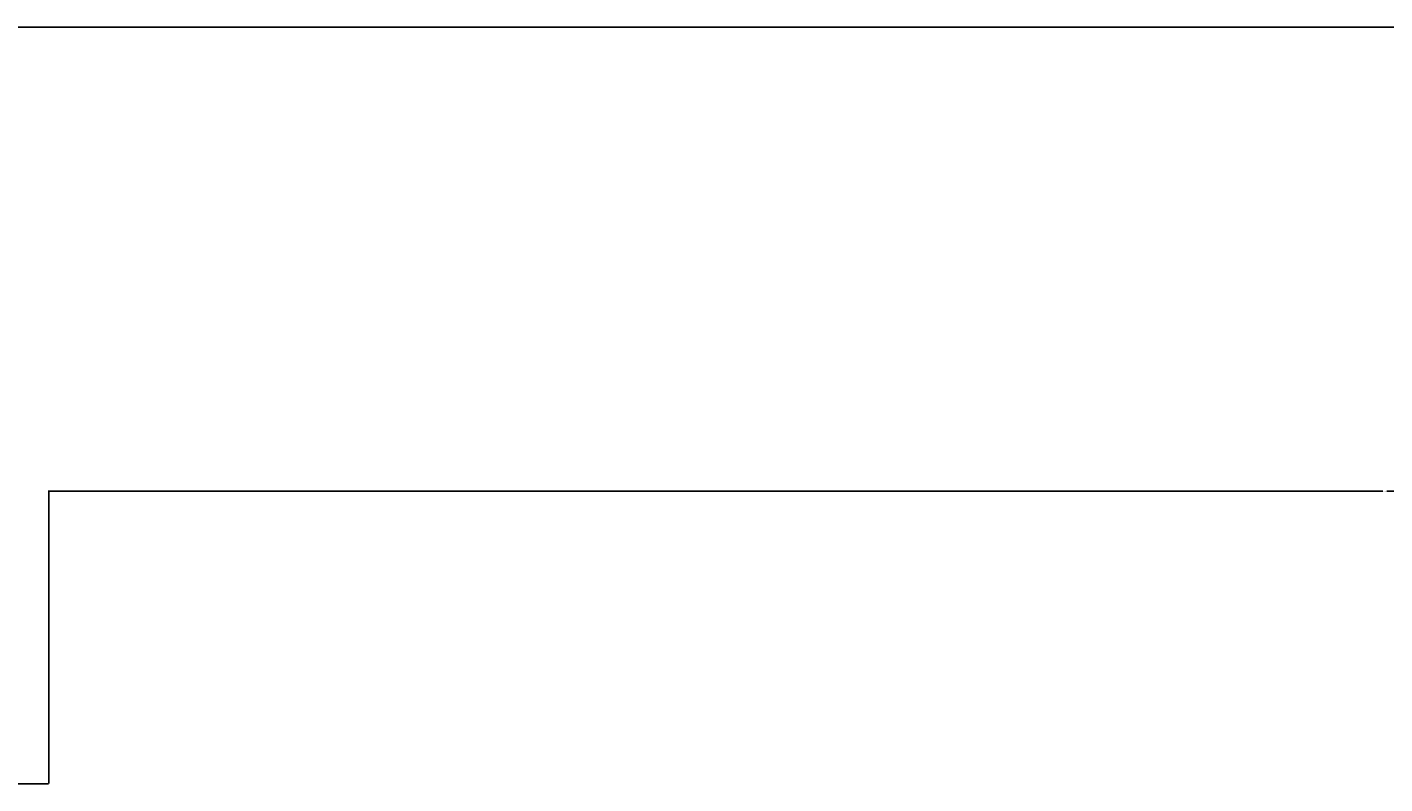
# Model space of a CAD drawing. Units: inches. Extents: x 2168 to 3056, y 1130 to 2629.
# Tile 32 of 42: x 2327 to 2598, y 2478 to 2629. Entities that reach past the tile are written whole.
import ezdxf

# ---------------------------------------------------------------- set-up
doc = ezdxf.new("R2010")
doc.units = ezdxf.units.IN
doc.layers.add('A-ANNO-DIMS', color=2, linetype='Continuous', lineweight=18)
doc.layers.add('A-ANNO-TTLB', color=7, linetype='Continuous', lineweight=25)
doc.styles.get("Standard").update_dxf_attribs({"font": 'arial.ttf'})
doc.dimstyles.get("Standard").update_dxf_attribs({"dimtxt": 0.18, "dimasz": 0.18, "dimexe": 0.18, "dimexo": 0.0625, "dimgap": 0.09, "dimtad": 0, "dimtih": 1, "dimtoh": 1, "dimdec": 4, "dimzin": 0, "dimdsep": 46, "dimtxsty": 'Standard', "dimcen": 0.09, "dimadec": 0, "dimazin": 0, "dimtfac": 1, "dimtdec": 4, "dimtofl": 0, "dimtmove": 0, "dimatfit": 3, "dimfxl": 1, "dimtolj": 1, "dimtzin": 0, "dimarcsym": 0})

# ---------------------------------------------------------------- blocks, each defined once
blk = doc.blocks.new('*D40')
at = {"layer": 'A-ANNO-DIMS', "color": 0, "lineweight": -2, "transparency": 16777216}
for p, q in [((2331.8, 2478.45), (2331.8, 2536.87)), ((2331.98, 2536.69), (2597.65, 2536.69)), ((2864.12, 2536.69), (2598.44, 2536.69)), ((2864.3, 2478.45), (2864.3, 2536.87))]:
    blk.add_line(p, q, dxfattribs=at)
at = {"layer": 'A-ANNO-DIMS', "color": 0, "transparency": 16777216}
for points in [[(2331.98, 2536.72), (2331.98, 2536.66), (2331.8, 2536.69)], [(2864.12, 2536.72), (2864.12, 2536.66), (2864.3, 2536.69)]]:
    blk.add_solid(points, dxfattribs=at)
at = {"layer": 'Defpoints', "color": 0, "transparency": 16777216}
for p in [(2864.3, 2536.69), (2331.8, 2478.39), (2864.3, 2478.39)]:
    blk.add_point(p, dxfattribs=at)
at = {"layer": 'A-ANNO-DIMS', "color": 0, "transparency": 16777216, "insert": (2598.05, 2536.69), "char_height": 0.18, "attachment_point": 5}
blk.add_mtext('\\A1;532.5', dxfattribs=at)
blk = doc.blocks.new('*D41')
at = {"layer": 'A-ANNO-DIMS', "color": 0, "lineweight": -2, "transparency": 16777216}
for p, q in [((2331.73, 2478.39), (2273.32, 2478.39)), ((2273.5, 2478.21), (2273.5, 1928.07)), ((2273.5, 1377.57), (2273.5, 1927.71)), ((2331.73, 1377.39), (2273.32, 1377.39))]:
    blk.add_line(p, q, dxfattribs=at)
at = {"layer": 'A-ANNO-DIMS', "color": 0, "transparency": 16777216}
for points in [[(2273.47, 2478.21), (2273.53, 2478.21), (2273.5, 2478.39)], [(2273.47, 1377.57), (2273.53, 1377.57), (2273.5, 1377.39)]]:
    blk.add_solid(points, dxfattribs=at)
at = {"layer": 'Defpoints', "color": 0, "transparency": 16777216}
for p in [(2273.5, 2478.39), (2331.8, 2478.39), (2331.8, 1377.39)]:
    blk.add_point(p, dxfattribs=at)
at = {"layer": 'A-ANNO-DIMS', "color": 0, "transparency": 16777216, "insert": (2273.5, 1927.89), "char_height": 0.18, "attachment_point": 5}
blk.add_mtext('\\A1;1101', dxfattribs=at)

msp = doc.modelspace()

# ---------------------------------------------------------------- linework, layer by layer
at = {"layer": 'A-ANNO-TTLB'}
msp.add_lwpolyline([(2168.16, 2629.19), (3055.63, 2629.19), (3055.63, 1130.19), (2168.16, 1130.19)], close=True, dxfattribs=at)

# ---------------------------------------------------------------- dimensions: what is measured, and where the dimension line sits
at = {"layer": 'A-ANNO-DIMS'}
dim = msp.add_linear_dim(base=(2864.3, 2536.69), p1=(2331.8, 2478.39), p2=(2864.3, 2478.39), dimstyle='Standard', override={"dimdec": 1, "dimlfac": 1, "dimrnd": 0, "dimzin": 0, "dimdsep": 46, "dimlunit": 2}, dxfattribs=at)
dim.commit()
dim.dimension.update_dxf_attribs({"geometry": '*D40', "text_midpoint": (2598.05, 2536.69)})
dim = msp.add_linear_dim(base=(2273.5, 2478.39), p1=(2331.8, 1377.39), p2=(2331.8, 2478.39), angle=90, dimstyle='Standard', override={"dimdec": 0, "dimlfac": 1, "dimrnd": 0, "dimzin": 0, "dimdsep": 46, "dimlunit": 2}, dxfattribs=at)
dim.commit()
dim.dimension.update_dxf_attribs({"geometry": '*D41', "text_midpoint": (2273.5, 1927.89)})

doc.saveas('drawing.dxf')
